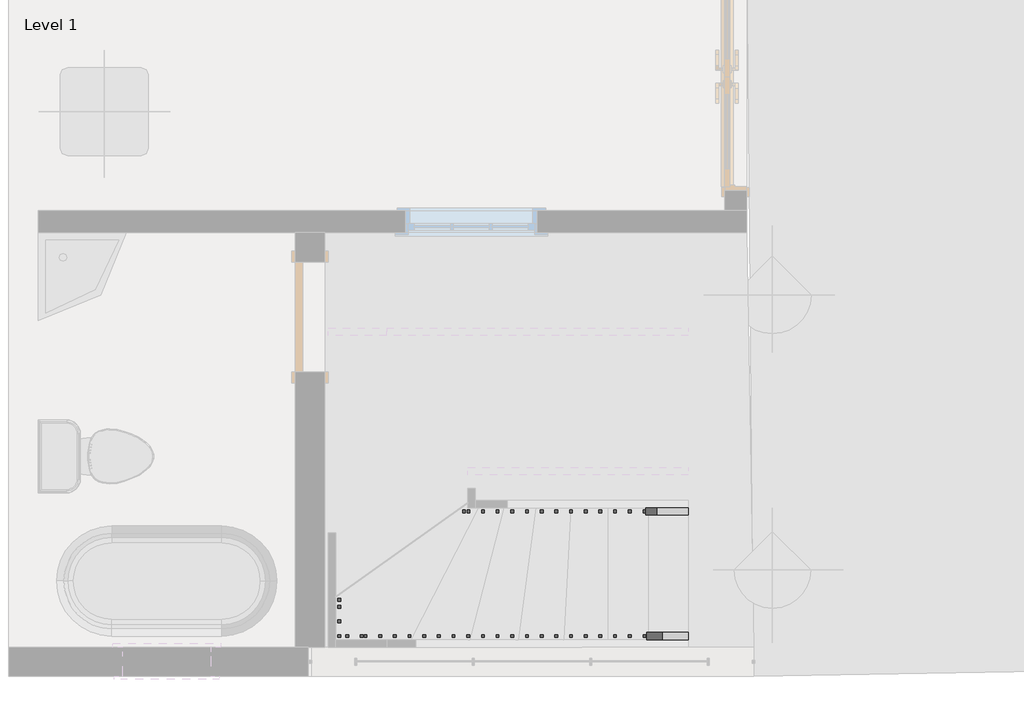
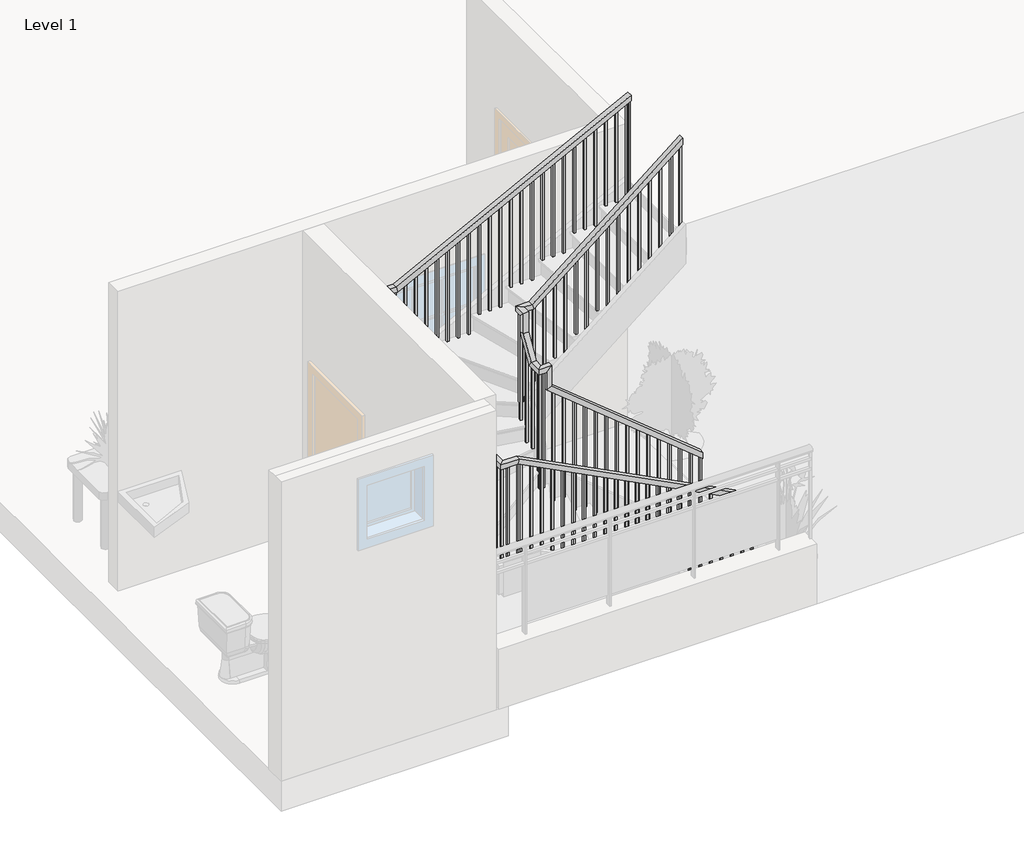
# One storey, part 2 of 3: 2 railings.
"""IFC4 building model written with IfcOpenShell, lengths in millimetres."""

from ifc_helpers import new_model, si_unit, frame, origin, place, context, project, spatial, polyline, outline, extrude, faceted_brep, element, save

model = new_model("IFC4")

# Units and contexts
model_context = context("Model", 3, world=origin())
ifc_project = project(units=[si_unit("LENGTHUNIT", "METRE", prefix="MILLI")], contexts=[model_context])

# Site, building, storey
site = spatial("IfcSite", under=ifc_project)
building = spatial("IfcBuilding", under=site)
storey = spatial("IfcBuildingStorey", under=building, Name="Level 1", Elevation=0.0)

# Railings
placement = place(None, origin())
element("IfcRailing", 1, ObjectType="Handrail - Rectangular", at=placement, inside=storey, context=model_context, shape_type="SolidModel", body=[
    faceted_brep([(-8055.8175858, 247.553629, 1025.2529681), (-8055.8175858, 247.553629, 959.7067088), (-8055.8175858, 298.353629, 959.7067088), (-8055.8175858, 298.353629, 1025.2529681), (-9507.3492777, 247.553629, 2208.7848338), (-9558.1492777, 247.553629, 2184.659247), (-9558.1492777, 298.353629, 2184.659247), (-9507.3492777, 298.353629, 2208.7848338), (-9507.3492777, 247.553629, 2414.6281882), (-9558.1492777, 247.553629, 2363.8281882), (-9558.1492777, 298.353629, 2363.8281882), (-9507.3492777, 298.353629, 2414.6281882), (-9634.3492777, 247.553629, 2414.6281882), (-9634.3492777, 247.553629, 2363.8281882), (-9583.5492777, 298.353629, 2363.8281882), (-9583.5492777, 298.353629, 2414.6281882), (-9634.3492777, 374.553629, 2414.6281882), (-9634.3492777, 403.6749629, 2363.8281882), (-9583.5492777, 403.6749629, 2363.8281882), (-9583.5492777, 374.553629, 2414.6281882), (-9634.3492777, 501.553629, 2631.5051451), (-9634.3492777, 552.353629, 2617.7256424), (-9583.5492777, 552.353629, 2617.7256424), (-9583.5492777, 501.553629, 2631.5051451), (-9634.3492777, 501.553629, 2837.3484995), (-9634.3492777, 552.353629, 2786.5484995), (-9583.5492777, 552.353629, 2786.5484995), (-9583.5492777, 501.553629, 2837.3484995), (-9634.3492777, 628.553629, 2837.3484995), (-9634.3492777, 628.553629, 2786.5484995), (-9583.5492777, 577.753629, 2786.5484995), (-9583.5492777, 577.753629, 2837.3484995), (-9507.3492777, 628.553629, 2837.3484995), (-9489.2638646, 628.553629, 2786.5484995), (-9489.2638646, 577.753629, 2786.5484995), (-9507.3492777, 577.753629, 2837.3484995), (-8055.8175858, 628.553629, 4020.8803652), (-8055.8175858, 577.753629, 4020.8803652), (-8055.8175858, 577.753629, 3955.3341059), (-8055.8175858, 628.553629, 3955.3341059)], [[[0, 1, 2, 3]], [[1, 0, 4, 5]], [[2, 1, 5, 6]], [[3, 2, 6, 7]], [[0, 3, 7, 4]], [[5, 4, 8, 9]], [[6, 5, 9, 10]], [[7, 6, 10, 11]], [[4, 7, 11, 8]], [[9, 8, 12, 13]], [[10, 9, 13, 14]], [[11, 10, 14, 15]], [[8, 11, 15, 12]], [[13, 12, 16, 17]], [[14, 13, 17, 18]], [[15, 14, 18, 19]], [[12, 15, 19, 16]], [[17, 16, 20, 21]], [[18, 17, 21, 22]], [[19, 18, 22, 23]], [[16, 19, 23, 20]], [[21, 20, 24, 25]], [[22, 21, 25, 26]], [[23, 22, 26, 27]], [[20, 23, 27, 24]], [[25, 24, 28, 29]], [[26, 25, 29, 30]], [[27, 26, 30, 31]], [[24, 27, 31, 28]], [[29, 28, 32, 33]], [[30, 29, 33, 34]], [[31, 30, 34, 35]], [[28, 31, 35, 32]], [[36, 37, 38, 39]], [[33, 32, 36, 39]], [[34, 33, 39, 38]], [[35, 34, 38, 37]], [[32, 35, 37, 36]]]),
    extrude(outline(polyline([(3881.7558784, -8146.0569213), (3866.2231262, -8165.1069213), (2878.6666667, -8165.1069213), (2878.6666667, -8146.0569213), (3881.7558784, -8146.0569213)])), frame((0.0, 593.628629, 0.0), z_axis=(0.0, 1.0, 0.0), x_axis=(0.0, 0.0, 1.0)), (0.0, 0.0, 1.0), 19.05),
    extrude(outline(polyline([(3798.9145334, -8247.6569213), (3783.3817813, -8266.7069213), (2878.6666667, -8266.7069213), (2878.6666667, -8247.6569213), (3798.9145334, -8247.6569213)])), frame((0.0, 593.628629, 0.0), z_axis=(0.0, 1.0, 0.0), x_axis=(0.0, 0.0, 1.0)), (0.0, 0.0, 1.0), 19.05),
    extrude(outline(polyline([(3716.0731885, -8349.2569213), (3700.5404364, -8368.3069213), (2709.3333333, -8368.3069213), (2709.3333333, -8349.2569213), (3716.0731885, -8349.2569213)])), frame((0.0, 593.628629, 0.0), z_axis=(0.0, 1.0, 0.0), x_axis=(0.0, 0.0, 1.0)), (0.0, 0.0, 1.0), 19.05),
    extrude(outline(polyline([(3633.2318436, -8450.8569213), (3617.6990914, -8469.9069213), (2709.3333333, -8469.9069213), (2709.3333333, -8450.8569213), (3633.2318436, -8450.8569213)])), frame((0.0, 593.628629, 0.0), z_axis=(0.0, 1.0, 0.0), x_axis=(0.0, 0.0, 1.0)), (0.0, 0.0, 1.0), 19.05),
    extrude(outline(polyline([(3550.3904987, -8552.4569213), (3534.8577465, -8571.5069213), (2709.3333333, -8571.5069213), (2709.3333333, -8552.4569213), (3550.3904987, -8552.4569213)])), frame((0.0, 593.628629, 0.0), z_axis=(0.0, 1.0, 0.0), x_axis=(0.0, 0.0, 1.0)), (0.0, 0.0, 1.0), 19.05),
    extrude(outline(polyline([(3467.5491538, -8654.0569213), (3452.0164016, -8673.1069213), (2540.0, -8673.1069213), (2540.0, -8654.0569213), (3467.5491538, -8654.0569213)])), frame((0.0, 593.628629, 0.0), z_axis=(0.0, 1.0, 0.0), x_axis=(0.0, 0.0, 1.0)), (0.0, 0.0, 1.0), 19.05),
    extrude(outline(polyline([(3384.7078088, -8755.6569213), (3369.1750567, -8774.7069213), (2540.0, -8774.7069213), (2540.0, -8755.6569213), (3384.7078088, -8755.6569213)])), frame((0.0, 593.628629, 0.0), z_axis=(0.0, 1.0, 0.0), x_axis=(0.0, 0.0, 1.0)), (0.0, 0.0, 1.0), 19.05),
    extrude(outline(polyline([(3301.8664639, -8857.2569213), (3286.3337117, -8876.3069213), (2540.0, -8876.3069213), (2540.0, -8857.2569213), (3301.8664639, -8857.2569213)])), frame((0.0, 593.628629, 0.0), z_axis=(0.0, 1.0, 0.0), x_axis=(0.0, 0.0, 1.0)), (0.0, 0.0, 1.0), 19.05),
    extrude(outline(polyline([(3219.025119, -8958.8569213), (3203.4923668, -8977.9069213), (2370.6666667, -8977.9069213), (2370.6666667, -8958.8569213), (3219.025119, -8958.8569213)])), frame((0.0, 593.628629, 0.0), z_axis=(0.0, 1.0, 0.0), x_axis=(0.0, 0.0, 1.0)), (0.0, 0.0, 1.0), 19.05),
    extrude(outline(polyline([(3136.1837741, -9060.4569213), (3120.6510219, -9079.5069213), (2370.6666667, -9079.5069213), (2370.6666667, -9060.4569213), (3136.1837741, -9060.4569213)])), frame((0.0, 593.628629, 0.0), z_axis=(0.0, 1.0, 0.0), x_axis=(0.0, 0.0, 1.0)), (0.0, 0.0, 1.0), 19.05),
    extrude(outline(polyline([(3053.3424291, -9162.0569213), (3037.809677, -9181.1069213), (2201.3333333, -9181.1069213), (2201.3333333, -9162.0569213), (3053.3424291, -9162.0569213)])), frame((0.0, 593.628629, 0.0), z_axis=(0.0, 1.0, 0.0), x_axis=(0.0, 0.0, 1.0)), (0.0, 0.0, 1.0), 19.05),
    extrude(outline(polyline([(2970.5010842, -9263.6569213), (2954.9683321, -9282.7069213), (2201.3333333, -9282.7069213), (2201.3333333, -9263.6569213), (2970.5010842, -9263.6569213)])), frame((0.0, 593.628629, 0.0), z_axis=(0.0, 1.0, 0.0), x_axis=(0.0, 0.0, 1.0)), (0.0, 0.0, 1.0), 19.05),
    extrude(outline(polyline([(2887.6597393, -9365.2569213), (2872.1269871, -9384.3069213), (2032.0, -9384.3069213), (2032.0, -9365.2569213), (2887.6597393, -9365.2569213)])), frame((0.0, 593.628629, 0.0), z_axis=(0.0, 1.0, 0.0), x_axis=(0.0, 0.0, 1.0)), (0.0, 0.0, 1.0), 19.05),
    extrude(outline(polyline([(2804.8183944, -9466.8569213), (2789.2856422, -9485.9069213), (2032.0, -9485.9069213), (2032.0, -9466.8569213), (2804.8183944, -9466.8569213)])), frame((0.0, 593.628629, 0.0), z_axis=(0.0, 1.0, 0.0), x_axis=(0.0, 0.0, 1.0)), (0.0, 0.0, 1.0), 19.05),
    extrude(outline(polyline([(481.4145328, 2496.5834745), (500.4645328, 2529.115018), (500.4645328, 1524.0), (481.4145328, 1524.0), (481.4145328, 2496.5834745)])), frame((-9618.4742777, 0.0, 0.0), z_axis=(1.0, 0.0, 0.0), x_axis=(0.0, 1.0, 0.0)), (0.0, 0.0, 1.0), 19.05),
    extrude(outline(polyline([(379.8145328, 2323.0819089), (398.8645328, 2355.6134525), (398.8645328, 1524.0), (379.8145328, 1524.0), (379.8145328, 2323.0819089)])), frame((-9618.4742777, 0.0, 0.0), z_axis=(1.0, 0.0, 0.0), x_axis=(0.0, 1.0, 0.0)), (0.0, 0.0, 1.0), 19.05),
    extrude(outline(polyline([(2111.7191617, -9468.6925858), (2127.2519138, -9487.7425858), (1016.0, -9487.7425858), (1016.0, -9468.6925858), (2111.7191617, -9468.6925858)])), frame((0.0, 263.428629, 0.0), z_axis=(0.0, 1.0, 0.0), x_axis=(0.0, 0.0, 1.0)), (0.0, 0.0, 1.0), 19.05),
    extrude(outline(polyline([(2028.8778167, -9367.0925858), (2044.4105689, -9386.1425858), (1016.0, -9386.1425858), (1016.0, -9367.0925858), (2028.8778167, -9367.0925858)])), frame((0.0, 263.428629, 0.0), z_axis=(0.0, 1.0, 0.0), x_axis=(0.0, 0.0, 1.0)), (0.0, 0.0, 1.0), 19.05),
    extrude(outline(polyline([(1946.0364718, -9265.4925858), (1961.569224, -9284.5425858), (846.6666667, -9284.5425858), (846.6666667, -9265.4925858), (1946.0364718, -9265.4925858)])), frame((0.0, 263.428629, 0.0), z_axis=(0.0, 1.0, 0.0), x_axis=(0.0, 0.0, 1.0)), (0.0, 0.0, 1.0), 19.05),
    extrude(outline(polyline([(1863.1951269, -9163.8925858), (1878.7278791, -9182.9425858), (846.6666667, -9182.9425858), (846.6666667, -9163.8925858), (1863.1951269, -9163.8925858)])), frame((0.0, 263.428629, 0.0), z_axis=(0.0, 1.0, 0.0), x_axis=(0.0, 0.0, 1.0)), (0.0, 0.0, 1.0), 19.05),
    extrude(outline(polyline([(1780.353782, -9062.2925858), (1795.8865341, -9081.3425858), (677.3333333, -9081.3425858), (677.3333333, -9062.2925858), (1780.353782, -9062.2925858)])), frame((0.0, 263.428629, 0.0), z_axis=(0.0, 1.0, 0.0), x_axis=(0.0, 0.0, 1.0)), (0.0, 0.0, 1.0), 19.05),
    extrude(outline(polyline([(1697.5124371, -8960.6925858), (1713.0451892, -8979.7425858), (677.3333333, -8979.7425858), (677.3333333, -8960.6925858), (1697.5124371, -8960.6925858)])), frame((0.0, 263.428629, 0.0), z_axis=(0.0, 1.0, 0.0), x_axis=(0.0, 0.0, 1.0)), (0.0, 0.0, 1.0), 19.05),
    extrude(outline(polyline([(1614.6710921, -8859.0925858), (1630.2038443, -8878.1425858), (508.0, -8878.1425858), (508.0, -8859.0925858), (1614.6710921, -8859.0925858)])), frame((0.0, 263.428629, 0.0), z_axis=(0.0, 1.0, 0.0), x_axis=(0.0, 0.0, 1.0)), (0.0, 0.0, 1.0), 19.05),
    extrude(outline(polyline([(1531.8297472, -8757.4925858), (1547.3624994, -8776.5425858), (508.0, -8776.5425858), (508.0, -8757.4925858), (1531.8297472, -8757.4925858)])), frame((0.0, 263.428629, 0.0), z_axis=(0.0, 1.0, 0.0), x_axis=(0.0, 0.0, 1.0)), (0.0, 0.0, 1.0), 19.05),
    extrude(outline(polyline([(1448.9884023, -8655.8925858), (1464.5211545, -8674.9425858), (508.0, -8674.9425858), (508.0, -8655.8925858), (1448.9884023, -8655.8925858)])), frame((0.0, 263.428629, 0.0), z_axis=(0.0, 1.0, 0.0), x_axis=(0.0, 0.0, 1.0)), (0.0, 0.0, 1.0), 19.05),
    extrude(outline(polyline([(1366.1470574, -8554.2925858), (1381.6798095, -8573.3425858), (338.6666667, -8573.3425858), (338.6666667, -8554.2925858), (1366.1470574, -8554.2925858)])), frame((0.0, 263.428629, 0.0), z_axis=(0.0, 1.0, 0.0), x_axis=(0.0, 0.0, 1.0)), (0.0, 0.0, 1.0), 19.05),
    extrude(outline(polyline([(1283.3057124, -8452.6925858), (1298.8384646, -8471.7425858), (338.6666667, -8471.7425858), (338.6666667, -8452.6925858), (1283.3057124, -8452.6925858)])), frame((0.0, 263.428629, 0.0), z_axis=(0.0, 1.0, 0.0), x_axis=(0.0, 0.0, 1.0)), (0.0, 0.0, 1.0), 19.05),
    extrude(outline(polyline([(1200.4643675, -8351.0925858), (1215.9971197, -8370.1425858), (338.6666667, -8370.1425858), (338.6666667, -8351.0925858), (1200.4643675, -8351.0925858)])), frame((0.0, 263.428629, 0.0), z_axis=(0.0, 1.0, 0.0), x_axis=(0.0, 0.0, 1.0)), (0.0, 0.0, 1.0), 19.05),
    extrude(outline(polyline([(1117.6230226, -8249.4925858), (1133.1557748, -8268.5425858), (169.3333333, -8268.5425858), (169.3333333, -8249.4925858), (1117.6230226, -8249.4925858)])), frame((0.0, 263.428629, 0.0), z_axis=(0.0, 1.0, 0.0), x_axis=(0.0, 0.0, 1.0)), (0.0, 0.0, 1.0), 19.05),
    extrude(outline(polyline([(1034.7816777, -8147.8925858), (1050.3144298, -8166.9425858), (169.3333333, -8166.9425858), (169.3333333, -8147.8925858), (1034.7816777, -8147.8925858)])), frame((0.0, 263.428629, 0.0), z_axis=(0.0, 1.0, 0.0), x_axis=(0.0, 0.0, 1.0)), (0.0, 0.0, 1.0), 19.05),
    extrude(outline(polyline([(-9587.5069213, 593.628629), (-9587.5069213, 612.678629), (-9568.4569213, 612.678629), (-9568.4569213, 593.628629), (-9587.5069213, 593.628629)])), frame((0.0, 0.0, 1862.6666667), z_axis=(0.0, 0.0, 1.0), x_axis=(1.0, 0.0, 0.0)), (0.0, 0.0, 1.0), 923.8818329),
    extrude(outline(polyline([(-9599.4242777, 593.628629), (-9618.4742777, 593.628629), (-9618.4742777, 612.678629), (-9599.4242777, 612.678629), (-9599.4242777, 593.628629)])), frame((0.0, 0.0, 1862.6666667), z_axis=(0.0, 0.0, 1.0), x_axis=(1.0, 0.0, 0.0)), (0.0, 0.0, 1.0), 923.8818329),
    extrude(outline(polyline([(-9599.4242777, 578.8427253), (-9618.4742777, 578.8427253), (-9618.4742777, 597.8927253), (-9599.4242777, 597.8927253), (-9599.4242777, 578.8427253)])), frame((0.0, 0.0, 1693.3333333), z_axis=(0.0, 0.0, 1.0), x_axis=(1.0, 0.0, 0.0)), (0.0, 0.0, 1.0), 1093.2151662),
    extrude(outline(polyline([(-9599.4242777, 278.2145328), (-9618.4742777, 278.2145328), (-9618.4742777, 297.2645328), (-9599.4242777, 297.2645328), (-9599.4242777, 278.2145328)])), frame((0.0, 0.0, 1354.6666667), z_axis=(0.0, 0.0, 1.0), x_axis=(1.0, 0.0, 0.0)), (0.0, 0.0, 1.0), 1009.1615215),
    extrude(outline(polyline([(-9599.4242777, 282.478629), (-9599.4242777, 263.428629), (-9618.4742777, 263.428629), (-9618.4742777, 282.478629), (-9599.4242777, 282.478629)])), frame((0.0, 0.0, 1185.3333333), z_axis=(0.0, 0.0, 1.0), x_axis=(1.0, 0.0, 0.0)), (0.0, 0.0, 1.0), 1178.4948549),
    extrude(outline(polyline([(-9568.4569213, 282.478629), (-9568.4569213, 263.428629), (-9587.5069213, 263.428629), (-9587.5069213, 282.478629), (-9568.4569213, 282.478629)])), frame((0.0, 0.0, 1185.3333333), z_axis=(0.0, 0.0, 1.0), x_axis=(1.0, 0.0, 0.0)), (0.0, 0.0, 1.0), 1178.4948549),
    extrude(outline(polyline([(3955.3341059, -8055.8175858), (3939.8013537, -8074.8675858), (2878.6666667, -8074.8675858), (2878.6666667, -8055.8175858), (3955.3341059, -8055.8175858)])), frame((0.0, 593.628629, 0.0), z_axis=(0.0, 1.0, 0.0), x_axis=(0.0, 0.0, 1.0)), (0.0, 0.0, 1.0), 19.05),
    extrude(outline(polyline([(959.7067088, -8055.8175858), (975.239461, -8074.8675858), (169.3333333, -8074.8675858), (169.3333333, -8055.8175858), (959.7067088, -8055.8175858)])), frame((0.0, 263.428629, 0.0), z_axis=(0.0, 1.0, 0.0), x_axis=(0.0, 0.0, 1.0)), (0.0, 0.0, 1.0), 19.05),
])
element("IfcRailing", 2, ObjectType="Handrail - Rectangular", at=placement, inside=storey, context=model_context, shape_type="SolidModel", body=[
    faceted_brep([(-8055.8175858, -616.046371, 1109.0771751), (-8055.8175858, -616.046371, 1051.9280057), (-8055.8175858, -565.246371, 1051.9280057), (-8055.8175858, -565.246371, 1109.0771751), (-10315.7994423, -616.046371, 2273.7644996), (-10328.1194936, -616.046371, 2222.9644996), (-10328.1194936, -565.246371, 2222.9644996), (-10315.7994423, -565.246371, 2273.7644996), (-10497.9492777, -616.046371, 2273.7644996), (-10497.9492777, -616.046371, 2222.9644996), (-10447.1492777, -565.246371, 2222.9644996), (-10447.1492777, -565.246371, 2273.7644996), (-10497.9492777, -338.8924184, 2273.7644996), (-10497.9492777, -330.9418422, 2222.9644996), (-10447.1492777, -330.9418422, 2222.9644996), (-10447.1492777, -338.8924184, 2273.7644996), (-10497.9492777, 1214.9996764, 2772.3688337), (-10497.9492777, 1222.9502525, 2721.5688337), (-10447.1492777, 1222.9502525, 2721.5688337), (-10447.1492777, 1214.9996764, 2772.3688337), (-10497.9492777, 1492.153629, 2721.5688337), (-10497.9492777, 1492.153629, 2772.3688337), (-10315.7994423, 1492.153629, 2772.3688337), (-10303.479391, 1492.153629, 2721.5688337), (-10447.1492777, 1441.353629, 2721.5688337), (-10303.479391, 1441.353629, 2721.5688337), (-10447.1492777, 1441.353629, 2772.3688337), (-10315.7994423, 1441.353629, 2772.3688337), (-8055.8175858, 1492.153629, 3937.0561582), (-8055.8175858, 1441.353629, 3937.0561582), (-8055.8175858, 1441.353629, 3879.9069889), (-8055.8175858, 1492.153629, 3879.9069889)], [[[0, 1, 2, 3]], [[1, 0, 4, 5]], [[2, 1, 5, 6]], [[3, 2, 6, 7]], [[0, 3, 7, 4]], [[5, 4, 8, 9]], [[6, 5, 9, 10]], [[7, 6, 10, 11]], [[4, 7, 11, 8]], [[9, 8, 12, 13]], [[10, 9, 13, 14]], [[11, 10, 14, 15]], [[8, 11, 15, 12]], [[13, 12, 16, 17]], [[14, 13, 17, 18]], [[15, 14, 18, 19]], [[12, 15, 19, 16]], [[20, 21, 22, 23]], [[24, 20, 23, 25]], [[26, 24, 25, 27]], [[21, 26, 27, 22]], [[17, 16, 21, 20]], [[18, 17, 20, 24]], [[19, 18, 24, 26]], [[16, 19, 26, 21]], [[28, 29, 30, 31]], [[23, 22, 28, 31]], [[25, 23, 31, 30]], [[27, 25, 30, 29]], [[22, 27, 29, 28]]]),
    extrude(outline(polyline([(3862.2268642, -8090.1244423), (2878.6666667, -8090.1244423), (2878.6666667, -8071.0744423), (3872.0443296, -8071.0744423), (3862.2268642, -8090.1244423)])), frame((0.0, 1457.228629, 0.0), z_axis=(0.0, 1.0, 0.0), x_axis=(0.0, 0.0, 1.0)), (0.0, 0.0, 1.0), 19.05),
    extrude(outline(polyline([(3809.8670491, -8191.7244423), (2878.6666667, -8191.7244423), (2878.6666667, -8172.6744423), (3819.6845145, -8172.6744423), (3809.8670491, -8191.7244423)])), frame((0.0, 1457.228629, 0.0), z_axis=(0.0, 1.0, 0.0), x_axis=(0.0, 0.0, 1.0)), (0.0, 0.0, 1.0), 19.05),
    extrude(outline(polyline([(3757.507234, -8293.3244423), (2878.6666667, -8293.3244423), (2878.6666667, -8274.2744423), (3767.3246993, -8274.2744423), (3757.507234, -8293.3244423)])), frame((0.0, 1457.228629, 0.0), z_axis=(0.0, 1.0, 0.0), x_axis=(0.0, 0.0, 1.0)), (0.0, 0.0, 1.0), 19.05),
    extrude(outline(polyline([(3705.1474189, -8394.9244423), (2709.3333333, -8394.9244423), (2709.3333333, -8375.8744423), (3714.9648842, -8375.8744423), (3705.1474189, -8394.9244423)])), frame((0.0, 1457.228629, 0.0), z_axis=(0.0, 1.0, 0.0), x_axis=(0.0, 0.0, 1.0)), (0.0, 0.0, 1.0), 19.05),
    extrude(outline(polyline([(3652.7876038, -8496.5244423), (2709.3333333, -8496.5244423), (2709.3333333, -8477.4744423), (3662.6050691, -8477.4744423), (3652.7876038, -8496.5244423)])), frame((0.0, 1457.228629, 0.0), z_axis=(0.0, 1.0, 0.0), x_axis=(0.0, 0.0, 1.0)), (0.0, 0.0, 1.0), 19.05),
    extrude(outline(polyline([(3600.4277887, -8598.1244423), (2709.3333333, -8598.1244423), (2709.3333333, -8579.0744423), (3610.245254, -8579.0744423), (3600.4277887, -8598.1244423)])), frame((0.0, 1457.228629, 0.0), z_axis=(0.0, 1.0, 0.0), x_axis=(0.0, 0.0, 1.0)), (0.0, 0.0, 1.0), 19.05),
    extrude(outline(polyline([(3548.0679735, -8699.7244423), (2540.0, -8699.7244423), (2540.0, -8680.6744423), (3557.8854389, -8680.6744423), (3548.0679735, -8699.7244423)])), frame((0.0, 1457.228629, 0.0), z_axis=(0.0, 1.0, 0.0), x_axis=(0.0, 0.0, 1.0)), (0.0, 0.0, 1.0), 19.05),
    extrude(outline(polyline([(3495.7081584, -8801.3244423), (2540.0, -8801.3244423), (2540.0, -8782.2744423), (3505.5256238, -8782.2744423), (3495.7081584, -8801.3244423)])), frame((0.0, 1457.228629, 0.0), z_axis=(0.0, 1.0, 0.0), x_axis=(0.0, 0.0, 1.0)), (0.0, 0.0, 1.0), 19.05),
    extrude(outline(polyline([(3443.3483433, -8902.9244423), (2540.0, -8902.9244423), (2540.0, -8883.8744423), (3453.1658086, -8883.8744423), (3443.3483433, -8902.9244423)])), frame((0.0, 1457.228629, 0.0), z_axis=(0.0, 1.0, 0.0), x_axis=(0.0, 0.0, 1.0)), (0.0, 0.0, 1.0), 19.05),
    extrude(outline(polyline([(3390.9885282, -9004.5244423), (2370.6666667, -9004.5244423), (2370.6666667, -8985.4744423), (3400.8059935, -8985.4744423), (3390.9885282, -9004.5244423)])), frame((0.0, 1457.228629, 0.0), z_axis=(0.0, 1.0, 0.0), x_axis=(0.0, 0.0, 1.0)), (0.0, 0.0, 1.0), 19.05),
    extrude(outline(polyline([(3338.6287131, -9106.1244423), (2370.6666667, -9106.1244423), (2370.6666667, -9087.0744423), (3348.4461784, -9087.0744423), (3338.6287131, -9106.1244423)])), frame((0.0, 1457.228629, 0.0), z_axis=(0.0, 1.0, 0.0), x_axis=(0.0, 0.0, 1.0)), (0.0, 0.0, 1.0), 19.05),
    extrude(outline(polyline([(3286.268898, -9207.7244423), (2370.6666667, -9207.7244423), (2370.6666667, -9188.6744423), (3296.0863633, -9188.6744423), (3286.268898, -9207.7244423)])), frame((0.0, 1457.228629, 0.0), z_axis=(0.0, 1.0, 0.0), x_axis=(0.0, 0.0, 1.0)), (0.0, 0.0, 1.0), 19.05),
    extrude(outline(polyline([(3233.9090828, -9309.3244423), (2201.3333333, -9309.3244423), (2201.3333333, -9290.2744423), (3243.7265482, -9290.2744423), (3233.9090828, -9309.3244423)])), frame((0.0, 1457.228629, 0.0), z_axis=(0.0, 1.0, 0.0), x_axis=(0.0, 0.0, 1.0)), (0.0, 0.0, 1.0), 19.05),
    extrude(outline(polyline([(3181.5492677, -9410.9244423), (2201.3333333, -9410.9244423), (2201.3333333, -9391.8744423), (3191.3667331, -9391.8744423), (3181.5492677, -9410.9244423)])), frame((0.0, 1457.228629, 0.0), z_axis=(0.0, 1.0, 0.0), x_axis=(0.0, 0.0, 1.0)), (0.0, 0.0, 1.0), 19.05),
    extrude(outline(polyline([(3129.1894526, -9512.5244423), (2201.3333333, -9512.5244423), (2201.3333333, -9493.4744423), (3139.0069179, -9493.4744423), (3129.1894526, -9512.5244423)])), frame((0.0, 1457.228629, 0.0), z_axis=(0.0, 1.0, 0.0), x_axis=(0.0, 0.0, 1.0)), (0.0, 0.0, 1.0), 19.05),
    extrude(outline(polyline([(3076.8296375, -9614.1244423), (2032.0, -9614.1244423), (2032.0, -9595.0744423), (3086.6471028, -9595.0744423), (3076.8296375, -9614.1244423)])), frame((0.0, 1457.228629, 0.0), z_axis=(0.0, 1.0, 0.0), x_axis=(0.0, 0.0, 1.0)), (0.0, 0.0, 1.0), 19.05),
    extrude(outline(polyline([(3024.4698224, -9715.7244423), (2032.0, -9715.7244423), (2032.0, -9696.6744423), (3034.2872877, -9696.6744423), (3024.4698224, -9715.7244423)])), frame((0.0, 1457.228629, 0.0), z_axis=(0.0, 1.0, 0.0), x_axis=(0.0, 0.0, 1.0)), (0.0, 0.0, 1.0), 19.05),
    extrude(outline(polyline([(2972.1100073, -9817.3244423), (2032.0, -9817.3244423), (2032.0, -9798.2744423), (2981.9274726, -9798.2744423), (2972.1100073, -9817.3244423)])), frame((0.0, 1457.228629, 0.0), z_axis=(0.0, 1.0, 0.0), x_axis=(0.0, 0.0, 1.0)), (0.0, 0.0, 1.0), 19.05),
    extrude(outline(polyline([(2919.7501921, -9918.9244423), (2032.0, -9918.9244423), (2032.0, -9899.8744423), (2929.5676575, -9899.8744423), (2919.7501921, -9918.9244423)])), frame((0.0, 1457.228629, 0.0), z_axis=(0.0, 1.0, 0.0), x_axis=(0.0, 0.0, 1.0)), (0.0, 0.0, 1.0), 19.05),
    extrude(outline(polyline([(2867.390377, -10020.5244423), (1862.6666667, -10020.5244423), (1862.6666667, -10001.4744423), (2877.2078424, -10001.4744423), (2867.390377, -10020.5244423)])), frame((0.0, 1457.228629, 0.0), z_axis=(0.0, 1.0, 0.0), x_axis=(0.0, 0.0, 1.0)), (0.0, 0.0, 1.0), 19.05),
    extrude(outline(polyline([(2815.0305619, -10122.1244423), (1862.6666667, -10122.1244423), (1862.6666667, -10103.0744423), (2824.8480272, -10103.0744423), (2815.0305619, -10122.1244423)])), frame((0.0, 1457.228629, 0.0), z_axis=(0.0, 1.0, 0.0), x_axis=(0.0, 0.0, 1.0)), (0.0, 0.0, 1.0), 19.05),
    extrude(outline(polyline([(2762.6707468, -10223.7244423), (1862.6666667, -10223.7244423), (1862.6666667, -10204.6744423), (2772.4882121, -10204.6744423), (2762.6707468, -10223.7244423)])), frame((0.0, 1457.228629, 0.0), z_axis=(0.0, 1.0, 0.0), x_axis=(0.0, 0.0, 1.0)), (0.0, 0.0, 1.0), 19.05),
    extrude(outline(polyline([(-10380.4742777, 1476.278629), (-10361.4242777, 1476.278629), (-10361.4242777, 1457.228629), (-10380.4742777, 1457.228629), (-10380.4742777, 1476.278629)])), frame((0.0, 0.0, 1862.6666667), z_axis=(0.0, 0.0, 1.0), x_axis=(1.0, 0.0, 0.0)), (0.0, 0.0, 1.0), 858.902167),
    extrude(outline(polyline([(-10482.0742777, 1408.6746764), (-10482.0742777, 1427.7246764), (-10463.0242777, 1427.7246764), (-10463.0242777, 1408.6746764), (-10482.0742777, 1408.6746764)])), frame((0.0, 0.0, 1862.6666667), z_axis=(0.0, 0.0, 1.0), x_axis=(1.0, 0.0, 0.0)), (0.0, 0.0, 1.0), 858.902167),
    extrude(outline(polyline([(-10482.0742777, 1307.0746764), (-10482.0742777, 1326.1246764), (-10463.0242777, 1326.1246764), (-10463.0242777, 1307.0746764), (-10482.0742777, 1307.0746764)])), frame((0.0, 0.0, 1862.6666667), z_axis=(0.0, 0.0, 1.0), x_axis=(1.0, 0.0, 0.0)), (0.0, 0.0, 1.0), 858.902167),
    extrude(outline(polyline([(1194.6325816, 2712.4824155), (1194.6325816, 1693.3333333), (1175.5825816, 1693.3333333), (1175.5825816, 2706.3697564), (1194.6325816, 2712.4824155)])), frame((-10482.0742777, 0.0, 0.0), z_axis=(1.0, 0.0, 0.0), x_axis=(0.0, 1.0, 0.0)), (0.0, 0.0, 1.0), 19.05),
    extrude(outline(polyline([(1093.0325816, 2679.8815673), (1093.0325816, 1693.3333333), (1073.9825816, 1693.3333333), (1073.9825816, 2673.7689082), (1093.0325816, 2679.8815673)])), frame((-10482.0742777, 0.0, 0.0), z_axis=(1.0, 0.0, 0.0), x_axis=(0.0, 1.0, 0.0)), (0.0, 0.0, 1.0), 19.05),
    extrude(outline(polyline([(991.4325816, 2647.280719), (991.4325816, 1693.3333333), (972.3825816, 1693.3333333), (972.3825816, 2641.16806), (991.4325816, 2647.280719)])), frame((-10482.0742777, 0.0, 0.0), z_axis=(1.0, 0.0, 0.0), x_axis=(0.0, 1.0, 0.0)), (0.0, 0.0, 1.0), 19.05),
    extrude(outline(polyline([(889.8325816, 2614.6798708), (889.8325816, 1693.3333333), (870.7825816, 1693.3333333), (870.7825816, 2608.5672118), (889.8325816, 2614.6798708)])), frame((-10482.0742777, 0.0, 0.0), z_axis=(1.0, 0.0, 0.0), x_axis=(0.0, 1.0, 0.0)), (0.0, 0.0, 1.0), 19.05),
    extrude(outline(polyline([(788.2325816, 2582.0790226), (788.2325816, 1693.3333333), (769.1825816, 1693.3333333), (769.1825816, 2575.9663635), (788.2325816, 2582.0790226)])), frame((-10482.0742777, 0.0, 0.0), z_axis=(1.0, 0.0, 0.0), x_axis=(0.0, 1.0, 0.0)), (0.0, 0.0, 1.0), 19.05),
    extrude(outline(polyline([(686.6325816, 2549.4781744), (686.6325816, 1693.3333333), (667.5825816, 1693.3333333), (667.5825816, 2543.3655153), (686.6325816, 2549.4781744)])), frame((-10482.0742777, 0.0, 0.0), z_axis=(1.0, 0.0, 0.0), x_axis=(0.0, 1.0, 0.0)), (0.0, 0.0, 1.0), 19.05),
    extrude(outline(polyline([(585.0325816, 2516.8773261), (585.0325816, 1524.0), (565.9825816, 1524.0), (565.9825816, 2510.7646671), (585.0325816, 2516.8773261)])), frame((-10482.0742777, 0.0, 0.0), z_axis=(1.0, 0.0, 0.0), x_axis=(0.0, 1.0, 0.0)), (0.0, 0.0, 1.0), 19.05),
    extrude(outline(polyline([(483.4325816, 2484.2764779), (483.4325816, 1524.0), (464.3825816, 1524.0), (464.3825816, 2478.1638189), (483.4325816, 2484.2764779)])), frame((-10482.0742777, 0.0, 0.0), z_axis=(1.0, 0.0, 0.0), x_axis=(0.0, 1.0, 0.0)), (0.0, 0.0, 1.0), 19.05),
    extrude(outline(polyline([(381.8325816, 2451.6756297), (381.8325816, 1524.0), (362.7825816, 1524.0), (362.7825816, 2445.5629706), (381.8325816, 2451.6756297)])), frame((-10482.0742777, 0.0, 0.0), z_axis=(1.0, 0.0, 0.0), x_axis=(0.0, 1.0, 0.0)), (0.0, 0.0, 1.0), 19.05),
    extrude(outline(polyline([(280.2325816, 2419.0747814), (280.2325816, 1524.0), (261.1825816, 1524.0), (261.1825816, 2412.9621224), (280.2325816, 2419.0747814)])), frame((-10482.0742777, 0.0, 0.0), z_axis=(1.0, 0.0, 0.0), x_axis=(0.0, 1.0, 0.0)), (0.0, 0.0, 1.0), 19.05),
    extrude(outline(polyline([(178.6325816, 2386.4739332), (178.6325816, 1354.6666667), (159.5825816, 1354.6666667), (159.5825816, 2380.3612742), (178.6325816, 2386.4739332)])), frame((-10482.0742777, 0.0, 0.0), z_axis=(1.0, 0.0, 0.0), x_axis=(0.0, 1.0, 0.0)), (0.0, 0.0, 1.0), 19.05),
    extrude(outline(polyline([(77.0325816, 2353.873085), (77.0325816, 1354.6666667), (57.9825816, 1354.6666667), (57.9825816, 2347.7604259), (77.0325816, 2353.873085)])), frame((-10482.0742777, 0.0, 0.0), z_axis=(1.0, 0.0, 0.0), x_axis=(0.0, 1.0, 0.0)), (0.0, 0.0, 1.0), 19.05),
    extrude(outline(polyline([(-24.5674184, 2321.2722368), (-24.5674184, 1354.6666667), (-43.6174184, 1354.6666667), (-43.6174184, 2315.1595777), (-24.5674184, 2321.2722368)])), frame((-10482.0742777, 0.0, 0.0), z_axis=(1.0, 0.0, 0.0), x_axis=(0.0, 1.0, 0.0)), (0.0, 0.0, 1.0), 19.05),
    extrude(outline(polyline([(-126.1674184, 2288.6713885), (-126.1674184, 1354.6666667), (-145.2174184, 1354.6666667), (-145.2174184, 2282.5587295), (-126.1674184, 2288.6713885)])), frame((-10482.0742777, 0.0, 0.0), z_axis=(1.0, 0.0, 0.0), x_axis=(0.0, 1.0, 0.0)), (0.0, 0.0, 1.0), 19.05),
    extrude(outline(polyline([(-227.7674184, 2256.0705403), (-227.7674184, 1354.6666667), (-246.8174184, 1354.6666667), (-246.8174184, 2249.9578813), (-227.7674184, 2256.0705403)])), frame((-10482.0742777, 0.0, 0.0), z_axis=(1.0, 0.0, 0.0), x_axis=(0.0, 1.0, 0.0)), (0.0, 0.0, 1.0), 19.05),
    extrude(outline(polyline([(-10482.0742777, -396.971371), (-10482.0742777, -377.921371), (-10463.0242777, -377.921371), (-10463.0242777, -396.971371), (-10482.0742777, -396.971371)])), frame((0.0, 0.0, 1185.3333333), z_axis=(0.0, 0.0, 1.0), x_axis=(1.0, 0.0, 0.0)), (0.0, 0.0, 1.0), 1037.6311663),
    extrude(outline(polyline([(-10482.0742777, -498.571371), (-10482.0742777, -479.521371), (-10463.0242777, -479.521371), (-10463.0242777, -498.571371), (-10482.0742777, -498.571371)])), frame((0.0, 0.0, 1185.3333333), z_axis=(0.0, 0.0, 1.0), x_axis=(1.0, 0.0, 0.0)), (0.0, 0.0, 1.0), 1037.6311663),
    extrude(outline(polyline([(-10407.8744423, -600.171371), (-10426.9244423, -600.171371), (-10426.9244423, -581.121371), (-10407.8744423, -581.121371), (-10407.8744423, -600.171371)])), frame((0.0, 0.0, 1185.3333333), z_axis=(0.0, 0.0, 1.0), x_axis=(1.0, 0.0, 0.0)), (0.0, 0.0, 1.0), 1037.6311663),
    extrude(outline(polyline([(2208.752671, -10300.5425858), (1185.3333333, -10300.5425858), (1185.3333333, -10281.4925858), (2198.9352056, -10281.4925858), (2208.752671, -10300.5425858)])), frame((0.0, -600.171371, 0.0), z_axis=(0.0, 1.0, 0.0), x_axis=(0.0, 0.0, 1.0)), (0.0, 0.0, 1.0), 19.05),
    extrude(outline(polyline([(2156.3928558, -10198.9425858), (1185.3333333, -10198.9425858), (1185.3333333, -10179.8925858), (2146.5753905, -10179.8925858), (2156.3928558, -10198.9425858)])), frame((0.0, -600.171371, 0.0), z_axis=(0.0, 1.0, 0.0), x_axis=(0.0, 0.0, 1.0)), (0.0, 0.0, 1.0), 19.05),
    extrude(outline(polyline([(2104.0330407, -10097.3425858), (1185.3333333, -10097.3425858), (1185.3333333, -10078.2925858), (2094.2155754, -10078.2925858), (2104.0330407, -10097.3425858)])), frame((0.0, -600.171371, 0.0), z_axis=(0.0, 1.0, 0.0), x_axis=(0.0, 0.0, 1.0)), (0.0, 0.0, 1.0), 19.05),
    extrude(outline(polyline([(2051.6732256, -9995.7425858), (1185.3333333, -9995.7425858), (1185.3333333, -9976.6925858), (2041.8557603, -9976.6925858), (2051.6732256, -9995.7425858)])), frame((0.0, -600.171371, 0.0), z_axis=(0.0, 1.0, 0.0), x_axis=(0.0, 0.0, 1.0)), (0.0, 0.0, 1.0), 19.05),
    extrude(outline(polyline([(1999.3134105, -9894.1425858), (1016.0, -9894.1425858), (1016.0, -9875.0925858), (1989.4959452, -9875.0925858), (1999.3134105, -9894.1425858)])), frame((0.0, -600.171371, 0.0), z_axis=(0.0, 1.0, 0.0), x_axis=(0.0, 0.0, 1.0)), (0.0, 0.0, 1.0), 19.05),
    extrude(outline(polyline([(1946.9535954, -9792.5425858), (1016.0, -9792.5425858), (1016.0, -9773.4925858), (1937.13613, -9773.4925858), (1946.9535954, -9792.5425858)])), frame((0.0, -600.171371, 0.0), z_axis=(0.0, 1.0, 0.0), x_axis=(0.0, 0.0, 1.0)), (0.0, 0.0, 1.0), 19.05),
    extrude(outline(polyline([(1894.5937803, -9690.9425858), (1016.0, -9690.9425858), (1016.0, -9671.8925858), (1884.7763149, -9671.8925858), (1894.5937803, -9690.9425858)])), frame((0.0, -600.171371, 0.0), z_axis=(0.0, 1.0, 0.0), x_axis=(0.0, 0.0, 1.0)), (0.0, 0.0, 1.0), 19.05),
    extrude(outline(polyline([(1842.2339651, -9589.3425858), (1016.0, -9589.3425858), (1016.0, -9570.2925858), (1832.4164998, -9570.2925858), (1842.2339651, -9589.3425858)])), frame((0.0, -600.171371, 0.0), z_axis=(0.0, 1.0, 0.0), x_axis=(0.0, 0.0, 1.0)), (0.0, 0.0, 1.0), 19.05),
    extrude(outline(polyline([(1789.87415, -9487.7425858), (846.6666667, -9487.7425858), (846.6666667, -9468.6925858), (1780.0566847, -9468.6925858), (1789.87415, -9487.7425858)])), frame((0.0, -600.171371, 0.0), z_axis=(0.0, 1.0, 0.0), x_axis=(0.0, 0.0, 1.0)), (0.0, 0.0, 1.0), 19.05),
    extrude(outline(polyline([(1737.5143349, -9386.1425858), (846.6666667, -9386.1425858), (846.6666667, -9367.0925858), (1727.6968696, -9367.0925858), (1737.5143349, -9386.1425858)])), frame((0.0, -600.171371, 0.0), z_axis=(0.0, 1.0, 0.0), x_axis=(0.0, 0.0, 1.0)), (0.0, 0.0, 1.0), 19.05),
    extrude(outline(polyline([(1685.1545198, -9284.5425858), (846.6666667, -9284.5425858), (846.6666667, -9265.4925858), (1675.3370545, -9265.4925858), (1685.1545198, -9284.5425858)])), frame((0.0, -600.171371, 0.0), z_axis=(0.0, 1.0, 0.0), x_axis=(0.0, 0.0, 1.0)), (0.0, 0.0, 1.0), 19.05),
    extrude(outline(polyline([(1632.7947047, -9182.9425858), (677.3333333, -9182.9425858), (677.3333333, -9163.8925858), (1622.9772393, -9163.8925858), (1632.7947047, -9182.9425858)])), frame((0.0, -600.171371, 0.0), z_axis=(0.0, 1.0, 0.0), x_axis=(0.0, 0.0, 1.0)), (0.0, 0.0, 1.0), 19.05),
    extrude(outline(polyline([(1580.4348896, -9081.3425858), (677.3333333, -9081.3425858), (677.3333333, -9062.2925858), (1570.6174242, -9062.2925858), (1580.4348896, -9081.3425858)])), frame((0.0, -600.171371, 0.0), z_axis=(0.0, 1.0, 0.0), x_axis=(0.0, 0.0, 1.0)), (0.0, 0.0, 1.0), 19.05),
    extrude(outline(polyline([(1528.0750744, -8979.7425858), (677.3333333, -8979.7425858), (677.3333333, -8960.6925858), (1518.2576091, -8960.6925858), (1528.0750744, -8979.7425858)])), frame((0.0, -600.171371, 0.0), z_axis=(0.0, 1.0, 0.0), x_axis=(0.0, 0.0, 1.0)), (0.0, 0.0, 1.0), 19.05),
    extrude(outline(polyline([(1475.7152593, -8878.1425858), (508.0, -8878.1425858), (508.0, -8859.0925858), (1465.897794, -8859.0925858), (1475.7152593, -8878.1425858)])), frame((0.0, -600.171371, 0.0), z_axis=(0.0, 1.0, 0.0), x_axis=(0.0, 0.0, 1.0)), (0.0, 0.0, 1.0), 19.05),
    extrude(outline(polyline([(1423.3554442, -8776.5425858), (508.0, -8776.5425858), (508.0, -8757.4925858), (1413.5379789, -8757.4925858), (1423.3554442, -8776.5425858)])), frame((0.0, -600.171371, 0.0), z_axis=(0.0, 1.0, 0.0), x_axis=(0.0, 0.0, 1.0)), (0.0, 0.0, 1.0), 19.05),
    extrude(outline(polyline([(1370.9956291, -8674.9425858), (508.0, -8674.9425858), (508.0, -8655.8925858), (1361.1781638, -8655.8925858), (1370.9956291, -8674.9425858)])), frame((0.0, -600.171371, 0.0), z_axis=(0.0, 1.0, 0.0), x_axis=(0.0, 0.0, 1.0)), (0.0, 0.0, 1.0), 19.05),
    extrude(outline(polyline([(1318.635814, -8573.3425858), (338.6666667, -8573.3425858), (338.6666667, -8554.2925858), (1308.8183486, -8554.2925858), (1318.635814, -8573.3425858)])), frame((0.0, -600.171371, 0.0), z_axis=(0.0, 1.0, 0.0), x_axis=(0.0, 0.0, 1.0)), (0.0, 0.0, 1.0), 19.05),
    extrude(outline(polyline([(1266.2759989, -8471.7425858), (338.6666667, -8471.7425858), (338.6666667, -8452.6925858), (1256.4585335, -8452.6925858), (1266.2759989, -8471.7425858)])), frame((0.0, -600.171371, 0.0), z_axis=(0.0, 1.0, 0.0), x_axis=(0.0, 0.0, 1.0)), (0.0, 0.0, 1.0), 19.05),
    extrude(outline(polyline([(1213.9161837, -8370.1425858), (338.6666667, -8370.1425858), (338.6666667, -8351.0925858), (1204.0987184, -8351.0925858), (1213.9161837, -8370.1425858)])), frame((0.0, -600.171371, 0.0), z_axis=(0.0, 1.0, 0.0), x_axis=(0.0, 0.0, 1.0)), (0.0, 0.0, 1.0), 19.05),
    extrude(outline(polyline([(1161.5563686, -8268.5425858), (169.3333333, -8268.5425858), (169.3333333, -8249.4925858), (1151.7389033, -8249.4925858), (1161.5563686, -8268.5425858)])), frame((0.0, -600.171371, 0.0), z_axis=(0.0, 1.0, 0.0), x_axis=(0.0, 0.0, 1.0)), (0.0, 0.0, 1.0), 19.05),
    extrude(outline(polyline([(1109.1965535, -8166.9425858), (169.3333333, -8166.9425858), (169.3333333, -8147.8925858), (1099.3790882, -8147.8925858), (1109.1965535, -8166.9425858)])), frame((0.0, -600.171371, 0.0), z_axis=(0.0, 1.0, 0.0), x_axis=(0.0, 0.0, 1.0)), (0.0, 0.0, 1.0), 19.05),
    extrude(outline(polyline([(-10325.3244423, 1476.278629), (-10306.2744423, 1476.278629), (-10306.2744423, 1457.228629), (-10325.3244423, 1457.228629), (-10325.3244423, 1476.278629)])), frame((0.0, 0.0, 1862.6666667), z_axis=(0.0, 0.0, 1.0), x_axis=(1.0, 0.0, 0.0)), (0.0, 0.0, 1.0), 858.902167),
    extrude(outline(polyline([(-10482.0742777, 1457.228629), (-10482.0742777, 1476.278629), (-10463.0242777, 1476.278629), (-10463.0242777, 1457.228629), (-10482.0742777, 1457.228629)])), frame((0.0, 0.0, 1862.6666667), z_axis=(0.0, 0.0, 1.0), x_axis=(1.0, 0.0, 0.0)), (0.0, 0.0, 1.0), 858.902167),
    extrude(outline(polyline([(1224.5246764, 2722.0740262), (1224.5246764, 1862.6666667), (1205.4746764, 1862.6666667), (1205.4746764, 2715.9613671), (1224.5246764, 2722.0740262)])), frame((-10482.0742777, 0.0, 0.0), z_axis=(1.0, 0.0, 0.0), x_axis=(0.0, 1.0, 0.0)), (0.0, 0.0, 1.0), 19.05),
    extrude(outline(polyline([(-10482.0742777, -348.4174184), (-10482.0742777, -329.3674184), (-10463.0242777, -329.3674184), (-10463.0242777, -348.4174184), (-10482.0742777, -348.4174184)])), frame((0.0, 0.0, 1185.3333333), z_axis=(0.0, 0.0, 1.0), x_axis=(1.0, 0.0, 0.0)), (0.0, 0.0, 1.0), 1037.6311663),
    extrude(outline(polyline([(-10463.0242777, -600.171371), (-10482.0742777, -600.171371), (-10482.0742777, -581.121371), (-10463.0242777, -581.121371), (-10463.0242777, -600.171371)])), frame((0.0, 0.0, 1185.3333333), z_axis=(0.0, 0.0, 1.0), x_axis=(1.0, 0.0, 0.0)), (0.0, 0.0, 1.0), 1037.6311663),
    extrude(outline(polyline([(2221.5240629, -10325.3244423), (1185.3333333, -10325.3244423), (1185.3333333, -10306.2744423), (2211.7065976, -10306.2744423), (2221.5240629, -10325.3244423)])), frame((0.0, -600.171371, 0.0), z_axis=(0.0, 1.0, 0.0), x_axis=(0.0, 0.0, 1.0)), (0.0, 0.0, 1.0), 19.05),
    extrude(outline(polyline([(3870.0895235, -8074.8675858), (2878.6666667, -8074.8675858), (2878.6666667, -8055.8175858), (3879.9069889, -8055.8175858), (3870.0895235, -8074.8675858)])), frame((0.0, 1457.228629, 0.0), z_axis=(0.0, 1.0, 0.0), x_axis=(0.0, 0.0, 1.0)), (0.0, 0.0, 1.0), 19.05),
    extrude(outline(polyline([(1061.7454711, -8074.8675858), (169.3333333, -8074.8675858), (169.3333333, -8055.8175858), (1051.9280057, -8055.8175858), (1061.7454711, -8074.8675858)])), frame((0.0, -600.171371, 0.0), z_axis=(0.0, 1.0, 0.0), x_axis=(0.0, 0.0, 1.0)), (0.0, 0.0, 1.0), 19.05),
])

save(model, "model.ifc")

# Revit data of these elements
# Type "Handrail - Rectangular"
#   Assembly Code = "C2010400"
#   built-in parameter 1008612 = 0.0416667 (stored number, unit not read)
#   built-in parameter 1008611 = 0.0416667 (stored number, unit not read)
#   built-in parameter 1008609 = 0.333333 (stored number, unit not read)
#   built-in parameter 1008604 = 0.166667 (stored number, unit not read)
#   built-in parameter 1008603 = 0.166667 (stored number, unit not read)
#   Railing Height = 3' - 0"
#   built-in parameter 1008630 = 2
#   built-in parameter 1008610 = 2
#   built-in parameter 1008618 = Baluster - Square : 3/4"
# Elements 1, 2 (IfcRailing, "Handrail - Rectangular")
#   Phase Created = New Construction
